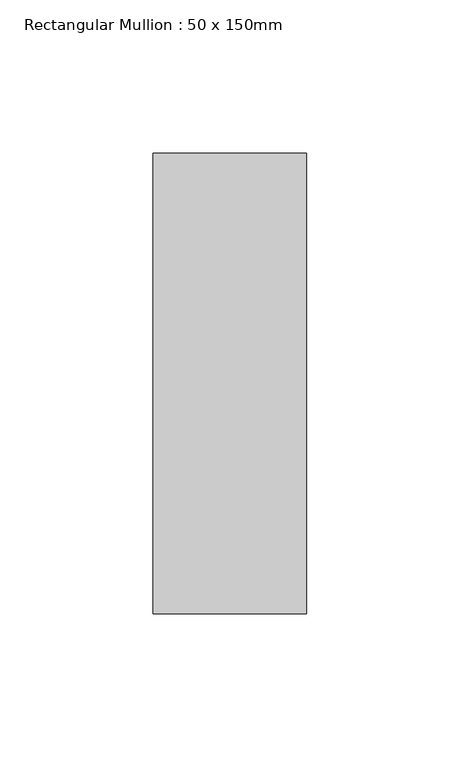
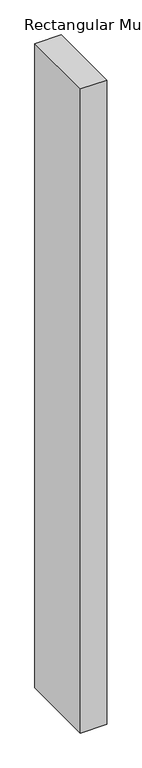
"""IFC4 building model written with IfcOpenShell, lengths in millimetres: member geometry, Rectangular Mullion : 50 x 150mm."""

from ifc_helpers import new_model, si_unit, frame, origin, place, context, project, spatial, polyline, outline, extrude, source, transform, mapped, element, save


def rectangular_mullion_50_x_150mm_817551cd(model_context):
    return source(origin(), model_context, "Body", "SweptSolid", [
        extrude(outline(polyline([(0.0, 75.0), (0.0, -75.0), (-50.0, -75.0), (-50.0, 75.0), (0.0, 75.0)])), frame((0.0, 0.0, -1296.6), z_axis=(0.0, 0.0, 1.0), x_axis=(1.0, 0.0, 0.0)), (0.0, 0.0, 1.0), 1296.6),
    ])


if __name__ == "__main__":
    model = new_model("IFC4")
    model_context = context("Model", 3, world=origin())
    ifc_project = project(units=[si_unit("LENGTHUNIT", "METRE", prefix="MILLI")], contexts=[model_context])
    site = spatial("IfcSite", under=ifc_project)
    building = spatial("IfcBuilding", under=site)
    placement = place(None, origin())
    rectangular_mullion_50_x_150mm_shape = rectangular_mullion_50_x_150mm_817551cd(model_context)
    element("IfcMember", 1, ObjectType="Rectangular Mullion : 50 x 150mm", at=placement, inside=building, context=model_context, shape_type="MappedRepresentation", body=[
        mapped(rectangular_mullion_50_x_150mm_shape, transform((0.0, 0.0, 0.0), x_axis=(1.0, 0.0, 0.0), y_axis=(0.0, 1.0, 0.0), z_axis=(0.0, 0.0, 1.0))),
    ])
    save(model, "model.ifc")

# Revit data of these elements
# Type "Rectangular Mullion : 50 x 150mm"
#   built-in parameter 1007304 = 0.492126 (stored number, unit not read)
#   built-in parameter 1007301 = 0.082021 (stored number, unit not read)
#   built-in parameter 1007300 = 0.082021 (stored number, unit not read)
# Element 1 (IfcMember, "Rectangular Mullion : 50 x 150mm")
#   Materials on its faces: "Aluminium"
# Materials
#   "Aluminium": class "Metal", colour RGB 247 247 247, transparency 0, Description = "Aluminium 6061", Cost = 0
